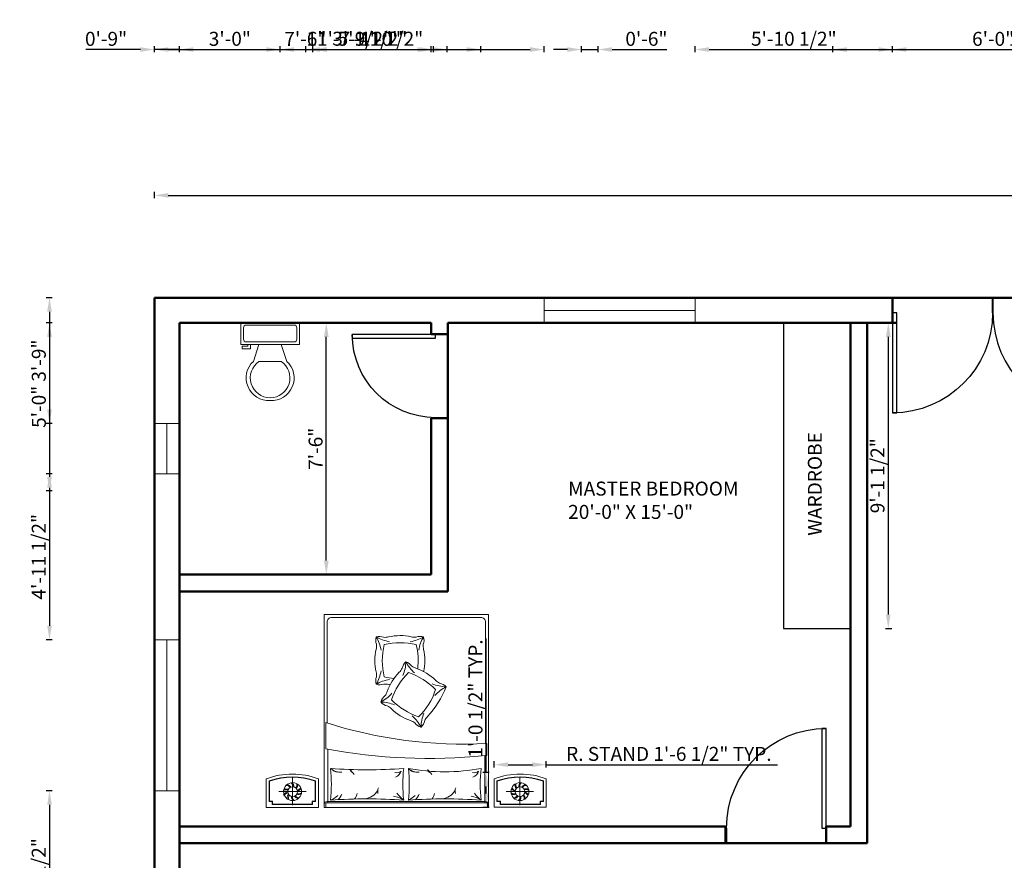
# Model space of a CAD drawing. Units: inches. Extents: x -46 to 764, y -530 to 112.
# Tile 2 of 5: x -46 to 307, y -188 to 112. Entities that reach past the tile are written whole.
import ezdxf

# ---------------------------------------------------------------- set-up
doc = ezdxf.new("R2010")
doc.units = ezdxf.units.IN
for name, color, linetype, lineweight in [('A-ANNO-DIMS', 2, 'Continuous', 18), ('A-AREA-IDEN', 7, 'Continuous', 18), ('A-DOOR', 3, 'Continuous', 25), ('A-FLOR-CASE', 32, 'Continuous', 25), ('A-FLOR-FIXT', 8, 'Continuous', 18), ('A-GLAZ', 4, 'Continuous', 18), ('A-WALL', 7, 'Continuous', 50), ('furn', 28, 'Continuous', 18), ('txt', 167, 'Continuous', 18)]:
    doc.layers.add(name, color=color, linetype=linetype, lineweight=lineweight)
doc.styles.get("Standard").update_dxf_attribs({"font": 'arial.ttf'})
doc.dimstyles.new('ISO-25', dxfattribs={"dimtxt": 5, "dimasz": 5, "dimexe": 1.25, "dimexo": 0.625, "dimtad": 1, "dimlunit": 3, "dimtxsty": 'Standard', "dimcen": 2.5, "dimadec": 0, "dimazin": 0, "dimtfac": 1, "dimtmove": 0, "dimatfit": 3, "dimfxl": 1, "dimfxlon": 1, "dimarcsym": 0})

# ---------------------------------------------------------------- blocks, each defined once
blk = doc.blocks.new('*U2')
for p, q in [((0, 0), (0, -6)), ((40, 0), (40, -6))]:
    blk.add_line(p, q)
blk.add_lwpolyline([(0, 0), (0, 40), (1.75, 40), (1.75, 0)], close=True)
blk.add_arc((0, 0), 40, 0, 90)
blk = doc.blocks.new('*U4')
for p, q in [((9.5, -6), (9.5, -2)), ((-10, -8.5), (-8, -8.5)), ((-10, -9.5), (-10, -8.5)), ((-7, -9.5), (-10, -9.5)), ((-8, -8.5), (-8, -8)), ((-7, -8), (-7, -9.5)), ((-4, -8), (-6, -14)), ((4, -8), (6, -14)), ((4, -14), (-4, -14))]:
    blk.add_line(p, q)
blk.add_lwpolyline([(10.5, -8), (10.5, 0), (-10.5, 0), (-10.5, -8)], close=True)
for points in [[(-9.5, -2), (-9.5, -6)], [(8.5, -1), (-8.5, -1)], [(-8.5, -7), (8.5, -7)]]:
    blk.add_lwpolyline(points)
for centre, radius, start, end in [((-8.625, -1.875), 0.8839, 81.8699, 188.1301), ((8.625, -1.875), 0.8839, 351.8699, 98.1301), ((-8.625, -6.125), 0.8839, 171.869898, 278.1301), ((8.625, -6.125), 0.8839, 261.8699, 8.1301), ((-0.4772, -19.9188), 8.0953, 133.01722, 273.38), ((0.0374, -19.8731), 7.127, 124.50543, 269.7), ((-0.0373, -19.8731), 7.127, 270.3, 55.4946), ((0.4773, -19.9188), 8.0953, 266.62, 46.9828)]:
    blk.add_arc(centre, radius, start, end)
blk = doc.blocks.new('*D10')
at = {"layer": 'A-ANNO-DIMS', "color": 0, "lineweight": -2, "transparency": 16777216}
for p, q in [((2.62, 48.57), (2.62, 50.82)), ((7.62, 49.57), (717.62, 49.57)), ((722.62, 48.57), (722.62, 50.82))]:
    blk.add_line(p, q, dxfattribs=at)
at = {"layer": 'A-ANNO-DIMS', "color": 0, "transparency": 16777216}
for points in [[(7.62, 50.4), (7.62, 48.73), (2.62, 49.57)], [(717.62, 50.4), (717.62, 48.73), (722.62, 49.57)]]:
    blk.add_solid(points, dxfattribs=at)
at = {"layer": 'Defpoints', "color": 0, "transparency": 16777216}
for p in [(722.62, 49.57), (2.62, 12.97), (722.62, 12.97)]:
    blk.add_point(p, dxfattribs=at)
at = {"layer": 'A-ANNO-DIMS', "color": 0, "transparency": 16777216, "insert": (362.62, 52.74), "char_height": 5, "attachment_point": 5}
blk.add_mtext("60'", dxfattribs=at)
blk = doc.blocks.new('BED-DOUBLE')
for p, q in [((1.34, 1.59), (1.34, 20.76)), ((57.43, 1.59), (57.43, 18.55)), ((57.72, 2.1), (1.02, 2.1))]:
    blk.add_line(p, q)
for points in [[(58.74, 0), (58.74, 68.93), (0, 68.93), (0, 0)], [(0.55, 0), (0.55, 1.59), (58.4, 1.59), (58.4, 0), (0, 0)]]:
    blk.add_lwpolyline(points)
for points in [[(57.72, 22.84), (57.72, 66.21, 0.414214), (56.03, 67.91), (2.72, 67.91, 0.414214), (1.02, 66.21), (1.02, 30.17)], [(18.6, 60.97, 0.159461), (18.72, 58.3, -0.076283), (18.6, 56.51, 0.115075), (18.6, 48.45, -0.076283), (18.72, 46.67, 0.159461), (18.6, 43.99)], [(20.35, 56.21, 0.091296), (18.6, 60.97, 0.091296), (23.37, 59.23)], [(30.8, 59.23, 0.091296), (35.58, 60.97, 0.091296), (33.82, 56.21, 0.091296)], [(32.9, 58.2, 0.111006), (21.48, 58.19, 0.119549), (21.48, 46.63, 0.033212), (24.99, 46.09)], [(29.21, 52.07, 0.159461), (27.9, 49.74, -0.076283), (26.85, 48.29, 0.115075), (22.59, 41.45, -0.076283), (21.75, 39.87, 0.159461), (20.23, 37.66)], [(28.18, 47.1, 0.091296), (29.21, 52.07, 0.091296), (32.34, 48.07)], [(23.37, 45.73, 0.091296), (18.6, 43.99, 0.091296), (20.35, 48.76, 0.091296)], [(39.88, 42.16, 0.111006), (30.18, 48.19, 0.119549), (24.07, 38.38, 0.107813), (33.74, 32.32)], [(38.65, 44.14, 0.091296), (43.62, 43.09, 0.091296), (39.61, 39.98, 0.091296)], [(25.2, 36.61, 0.091296), (20.23, 37.66, 0.091296), (24.24, 40.78, 0.091296)], [(33.79, 32.33, 0.121865), (39.88, 42.16, 0.121865)], [(35.68, 33.66, 0.091296), (34.64, 28.68, 0.091296), (31.51, 32.68, 0.091296)]]:
    blk.add_lwpolyline(points, format="xyb")
for points in [[(58.23, 18.55), (57.43, 18.55, -0.072944), (0.55, 20.92), (0.55, 30.34, 0.092568), (58.23, 22.87)], [(28.45, 13.91, 0.058596), (28.45, 2.57, 0.036648), (2.28, 2.57, 0.052163), (2.28, 13.91, 0.036967)], [(56.14, 13.91, 0.058596), (56.14, 2.57, 0.036889), (30.14, 2.57, 0.052163), (30.14, 13.91, 0.093111)]]:
    blk.add_lwpolyline(points, format="xyb", close=True)
for centre, radius, start, end in [((19.65, 56.16), 4.92, 70.7023, 102.284), ((21.76, 66.68), 5.9, 265.2252, 282.6741), ((27.14, 43.67), 17.74, 77.0576, 103.3153), ((32.37, 66.72), 5.9, 257.6988, 275.1477), ((34.43, 56.82), 4.3, 74.5791, 110.8198), ((31.43, 59.81), 4.3, 339.3666, 15.6073), ((9.55, 52.37), 24.07, 353.1956, 14.0284), ((41.33, 57.79), 5.9, 175.0387, 192.4877), ((18.3, 52.48), 17.74, 346.8711, 13.1289), ((27.56, 47.43), 4.92, 38.7754, 70.3571), ((34.92, 55.25), 5.9, 233.2983, 250.7472), ((27.31, 32.87), 17.74, 45.1307, 71.3884), ((19.87, 47.76), 3.97, 251.3996, 291.5774), ((21.86, 38.19), 5.9, 77.6988, 95.1477), ((27.09, 61.25), 17.74, 257.0576, 258.7033), ((9.2, 57.16), 37.18, 318.3818, 337.7644), ((43.94, 49.66), 5.9, 225.7718, 243.2208), ((40.46, 40.18), 4.3, 42.6522, 78.8929), ((23.3, 40.19), 3.97, 219.4726, 259.6505), ((19.93, 31.02), 5.9, 45.7718, 63.2208), ((36.56, 47.81), 17.74, 225.1307, 251.3884), ((41.21, 28.34), 5.9, 135.5854, 153.0343), ((28.95, 25.44), 5.9, 53.2983, 70.7472), ((35.78, 32.68), 4.15, 217.2937, 254.0973), ((31.74, 31.86), 4.3, 312.4658, 348.7065), ((4.9, 15.54), 2.94, 213.6349, 270.8456), ((5.76, 17.16), 4.64, 224.406, 276.8342), ((10.31, 13.43), 0.952, 173.7543, 257.2187), ((20.8, 21.81), 14.18, 216.2085, 225.0849), ((25.94, 14.96), 2.58, 256.4823, 308.5563), ((23.98, 14.17), 3.77, 294.2916, 340.9896), ((33.45, 17.16), 4.64, 224.406, 276.8342), ((32.59, 15.54), 2.94, 213.6349, 270.8456), ((38, 13.43), 0.952, 173.7543, 257.2187), ((48.49, 21.81), 14.18, 216.2085, 225.0849), ((53.63, 14.96), 2.58, 256.4823, 308.5563), ((51.67, 14.17), 3.77, 294.2916, 340.9896), ((-1.12, 10.34), 8.56, 294.6457, 314.1585), ((1.84, 6.34), 4.75, 310.5354, 340.3558), ((7.42, 5.72), 4.41, 321.8174, 349.8987), ((13.79, 9.29), 6.29, 276.6849, 328.3182), ((21.96, 5.79), 2.82, 155.8927, 196.1192), ((22.41, -6.92), 11.24, 57.5379, 77.5233), ((36.96, 13.18), 13.6, 216.4935, 231.2792), ((26.57, 10.34), 8.56, 294.6457, 314.1585), ((29.53, 6.34), 4.75, 310.5354, 340.3558), ((35.11, 5.72), 4.41, 321.8174, 349.8987), ((41.48, 9.29), 6.29, 276.6849, 328.3182), ((49.65, 5.79), 2.82, 155.8927, 196.1192), ((50.1, -6.92), 11.24, 57.5379, 77.5233), ((64.65, 13.18), 13.6, 216.4935, 231.2792), ((1.02, 1.08), 1.02, 90, 180), ((57.72, 1.08), 1.02, 0, 90)]:
    blk.add_arc(centre, radius, start, end)
blk = doc.blocks.new('NIGHTSTAND-L')
for p, q in [((9.43, 10.52), (9.43, 0.73)), ((4.54, 5.63), (14.33, 5.63))]:
    blk.add_line(p, q)
blk.add_lwpolyline([(0, 10.19), (0, 0), (18.68, 0), (18.68, 10.19, 0.181818)], format="xyb", close=True)
for points in [[(17.66, 2.14), (17.66, 9.48, 0.167087), (1.02, 9.48), (1.02, 2.14)], [(17.55, 2.14), (17.55, 9.4, 0.165559), (1.12, 9.4), (1.12, 2.14)]]:
    blk.add_lwpolyline(points, format="xyb")
for points in [[(2.24, 1.02), (2.24, 2.24), (1.02, 2.24)], [(2.14, 1.02), (2.14, 2.14), (1.02, 2.14)], [(2.14, 1.12), (16.54, 1.12)], [(2.14, 1.02), (16.54, 1.02)], [(16.43, 1.02), (16.43, 2.24), (17.66, 2.24)], [(16.54, 1.02), (16.54, 2.14), (17.66, 2.14)]]:
    blk.add_lwpolyline(points)
for radius in [3.2, 1.73]:
    blk.add_circle((9.43, 5.63), radius)
for centre, radius, start, end in [((7.17, 6.28), 1.57, 31.462, 91.6998), ((7.07, 6.1), 2.05, 33.5103, 79.83), ((7.98, 7.48), 1.57, 355.462, 55.6998), ((7.8, 7.4), 2.05, 357.5103, 43.83), ((9.35, 7.98), 1.57, 319.462, 19.6998), ((9.15, 8.02), 2.05, 321.5103, 7.83), ((10.75, 7.58), 1.57, 283.462, 343.6998), ((6.99, 4.73), 1.57, 67.462, 127.6998), ((7.01, 4.53), 2.05, 69.5103, 115.83), ((8.02, 3.43), 2.05, 105.5103, 151.83), ((7.89, 3.59), 1.57, 103.462, 163.6998), ((9.48, 3.14), 2.05, 141.5103, 187.83), ((9.52, 3.28), 1.57, 139.462, 199.6998), ((11.07, 3.86), 2.05, 177.5103, 223.83), ((10.88, 3.77), 1.57, 175.462, 235.6998), ((11.8, 5.16), 2.05, 213.5103, 259.83), ((11.7, 4.98), 1.57, 211.462, 271.6998), ((11.63, 6.64), 2.05, 249.5103, 295.83), ((11.64, 6.43), 1.57, 247.462, 307.6998), ((10.61, 7.73), 2.05, 285.5103, 331.83)]:
    blk.add_arc(centre, radius, start, end)
blk = doc.blocks.new('NIGHTSTAND-R')
for p, q in [((9.24, 10.52), (9.24, 0.73)), ((14.14, 5.62), (4.35, 5.62))]:
    blk.add_line(p, q)
blk.add_lwpolyline([(18.68, 10.19), (18.68, 0), (0, 0), (0, 10.19, -0.181818)], format="xyb", close=True)
for points in [[(1.02, 2.14), (1.02, 9.48, -0.167087), (17.66, 9.48), (17.66, 2.14)], [(1.12, 2.14), (1.12, 9.4, -0.165559), (17.56, 9.4), (17.56, 2.14)]]:
    blk.add_lwpolyline(points, format="xyb")
for points in [[(2.24, 1.02), (2.24, 2.24), (1.02, 2.24)], [(2.14, 1.02), (2.14, 2.14), (1.02, 2.14)], [(16.54, 1.12), (2.14, 1.12)], [(16.54, 1.02), (2.14, 1.02)], [(16.43, 1.02), (16.43, 2.24), (17.66, 2.24)], [(16.54, 1.02), (16.54, 2.14), (17.66, 2.14)]]:
    blk.add_lwpolyline(points)
for radius in [3.2, 1.73]:
    blk.add_circle((9.24, 5.62), radius)
for centre, radius, start, end in [((7.93, 7.57), 1.57, 196.3002, 256.538), ((9.52, 8.02), 2.05, 172.17, 218.4897), ((9.32, 7.97), 1.57, 160.3002, 220.538), ((10.88, 7.4), 2.05, 136.17, 182.4897), ((10.69, 7.48), 1.57, 124.3002, 184.538), ((11.61, 6.09), 2.05, 100.17, 146.4897), ((11.5, 6.27), 1.57, 88.3002, 148.538), ((7.03, 6.43), 1.57, 232.3002, 292.538), ((7.05, 6.63), 2.05, 244.17, 290.4897), ((8.06, 7.73), 2.05, 208.17, 254.4897), ((6.98, 4.98), 1.57, 268.3002, 328.538), ((6.88, 5.15), 2.05, 280.17, 326.4897), ((7.79, 3.77), 1.57, 304.3002, 4.538), ((7.6, 3.85), 2.05, 316.17, 2.4897), ((9.16, 3.27), 1.57, 340.3002, 40.538), ((8.96, 3.23), 2.05, 352.17, 38.4897), ((11.43, 4.61), 2.05, 64.17, 110.4897), ((11.45, 4.82), 1.57, 52.3002, 112.538), ((10.56, 3.67), 1.57, 16.3002, 76.538), ((10.42, 3.52), 2.05, 28.17, 74.4897)]:
    blk.add_arc(centre, radius, start, end)
blk = doc.blocks.new('WIN-54IN')
blk.add_line((4.5, 54), (4.5, 0))
blk.add_lwpolyline([(0, 54), (9, 54), (9, 0), (0, 0)], close=True)
blk = doc.blocks.new('WIN-18IN')
blk.add_line((4.5, 18), (4.5, 0))
blk.add_lwpolyline([(0, 18), (9, 18), (9, 0), (0, 0)], close=True)
blk = doc.blocks.new('*D31')
at = {"layer": 'A-ANNO-DIMS', "color": 0, "lineweight": -2, "transparency": 16777216}
for p, q in [((124.13, -154.98), (124.13, -152.73)), ((129.13, -153.98), (137.81, -153.98)), ((142.81, -154.98), (142.81, -152.73)), ((142.81, -153.98), (225.47, -153.98))]:
    blk.add_line(p, q, dxfattribs=at)
at = {"layer": 'A-ANNO-DIMS', "color": 0, "transparency": 16777216}
for points in [[(129.13, -153.14), (129.13, -154.81), (124.13, -153.98)], [(137.81, -153.14), (137.81, -154.81), (142.81, -153.98)]]:
    blk.add_solid(points, dxfattribs=at)
at = {"layer": 'Defpoints', "color": 0, "transparency": 16777216}
for p in [(142.81, -153.98), (124.13, -156.78), (142.81, -156.78)]:
    blk.add_point(p, dxfattribs=at)
at = {"layer": 'A-ANNO-DIMS', "color": 0, "transparency": 16777216, "insert": (186.64, -150.77), "char_height": 5, "attachment_point": 5}
blk.add_mtext('R. STAND 1\'-6 1/2" TYP.', dxfattribs=at)
blk = doc.blocks.new('*D32')
at = {"layer": 'A-ANNO-DIMS', "color": 0, "lineweight": -2, "transparency": 16777216}
for p, q in [((121.33, -156.78), (121.33, -108.87)), ((122.33, -156.78), (120.08, -156.78)), ((121.33, -164.23), (121.33, -161.78)), ((122.33, -169.23), (120.08, -169.23))]:
    blk.add_line(p, q, dxfattribs=at)
at = {"layer": 'A-ANNO-DIMS', "color": 0, "transparency": 16777216}
for points in [[(120.5, -161.78), (122.16, -161.78), (121.33, -156.78)], [(120.5, -164.23), (122.16, -164.23), (121.33, -169.23)]]:
    blk.add_solid(points, dxfattribs=at)
at = {"layer": 'Defpoints', "color": 0, "transparency": 16777216}
for p in [(121.33, -156.78), (124.13, -156.78), (124.13, -169.23)]:
    blk.add_point(p, dxfattribs=at)
at = {"layer": 'A-ANNO-DIMS', "color": 0, "transparency": 16777216, "insert": (118.12, -130.32), "char_height": 5, "attachment_point": 5, "rotation": 90}
blk.add_mtext('1\'-0 1/2" TYP.', dxfattribs=at)
blk = doc.blocks.new('*D43')
at = {"layer": 'A-ANNO-DIMS', "color": 0, "lineweight": -2, "transparency": 16777216}
for p, q in [((227.62, -503.53), (227.62, -505.78)), ((251.62, -503.53), (251.62, -505.78)), ((232.62, -504.53), (246.62, -504.53))]:
    blk.add_line(p, q, dxfattribs=at)
at = {"layer": 'A-ANNO-DIMS', "color": 0, "transparency": 16777216}
for points in [[(232.62, -503.7), (232.62, -505.36), (227.62, -504.53)], [(246.62, -503.7), (246.62, -505.36), (251.62, -504.53)]]:
    blk.add_solid(points, dxfattribs=at)
at = {"layer": 'Defpoints', "color": 0, "transparency": 16777216}
for p in [(227.62, -105.31), (251.62, -105.31), (251.62, -504.53)]:
    blk.add_point(p, dxfattribs=at)
at = {"layer": 'A-ANNO-DIMS', "color": 0, "transparency": 16777216, "insert": (239.62, -501.35), "char_height": 5, "attachment_point": 5}
blk.add_mtext('2\'-0"', dxfattribs=at)
blk = doc.blocks.new('*D44')
at = {"layer": 'A-ANNO-DIMS', "color": 0, "lineweight": -2, "transparency": 16777216}
for p, q in [((264.12, 3.97), (266.37, 3.97)), ((265.12, -1.03), (265.12, -100.31)), ((264.12, -105.31), (266.37, -105.31))]:
    blk.add_line(p, q, dxfattribs=at)
at = {"layer": 'A-ANNO-DIMS', "color": 0, "transparency": 16777216}
for points in [[(264.29, -1.03), (265.96, -1.03), (265.12, 3.97)], [(264.29, -100.31), (265.96, -100.31), (265.12, -105.31)]]:
    blk.add_solid(points, dxfattribs=at)
at = {"layer": 'Defpoints', "color": 0, "transparency": 16777216}
for p in [(227.62, 3.97), (227.62, -105.31), (265.12, -105.31)]:
    blk.add_point(p, dxfattribs=at)
at = {"layer": 'A-ANNO-DIMS', "color": 0, "transparency": 16777216, "insert": (261.91, -50.67), "char_height": 5, "attachment_point": 5, "rotation": 90}
blk.add_mtext('9\'-1 1/2"', dxfattribs=at)
blk = doc.blocks.new('*D45')
at = {"layer": 'A-ANNO-DIMS', "color": 0, "lineweight": -2, "transparency": 16777216}
for p, q in [((11.62, 100.72), (11.62, 102.97)), ((101.62, 100.72), (101.62, 102.97)), ((16.62, 101.72), (96.62, 101.72))]:
    blk.add_line(p, q, dxfattribs=at)
at = {"layer": 'A-ANNO-DIMS', "color": 0, "transparency": 16777216}
for points in [[(16.62, 102.55), (16.62, 100.88), (11.62, 101.72)], [(96.62, 102.55), (96.62, 100.88), (101.62, 101.72)]]:
    blk.add_solid(points, dxfattribs=at)
at = {"layer": 'Defpoints', "color": 0, "transparency": 16777216}
for p in [(101.62, 101.72), (11.62, -86.03), (101.62, -86.03)]:
    blk.add_point(p, dxfattribs=at)
at = {"layer": 'A-ANNO-DIMS', "color": 0, "transparency": 16777216, "insert": (56.62, 104.89), "char_height": 5, "attachment_point": 5}
blk.add_mtext('7\'-6"', dxfattribs=at)
blk = doc.blocks.new('*D46')
at = {"layer": 'A-ANNO-DIMS', "color": 0, "lineweight": -2, "transparency": 16777216}
for p, q in [((65.12, 3.97), (62.87, 3.97)), ((64.12, -81.03), (64.12, -1.03)), ((65.12, -86.03), (62.87, -86.03))]:
    blk.add_line(p, q, dxfattribs=at)
at = {"layer": 'A-ANNO-DIMS', "color": 0, "transparency": 16777216}
for points in [[(63.29, -1.03), (64.96, -1.03), (64.12, 3.97)], [(63.29, -81.03), (64.96, -81.03), (64.12, -86.03)]]:
    blk.add_solid(points, dxfattribs=at)
at = {"layer": 'Defpoints', "color": 0, "transparency": 16777216}
for p in [(64.12, 3.97), (101.62, 3.97), (101.62, -86.03)]:
    blk.add_point(p, dxfattribs=at)
at = {"layer": 'A-ANNO-DIMS', "color": 0, "transparency": 16777216, "insert": (60.95, -41.03), "char_height": 5, "attachment_point": 5, "rotation": 90}
blk.add_mtext('7\'-6"', dxfattribs=at)
blk = doc.blocks.new('*D48')
at = {"layer": 'A-ANNO-DIMS', "color": 0, "lineweight": -2, "transparency": 16777216}
for p, q in [((-33.88, 3.97), (-36.13, 3.97)), ((-34.88, -1.03), (-34.88, -51.03)), ((-33.88, -56.03), (-36.13, -56.03))]:
    blk.add_line(p, q, dxfattribs=at)
at = {"layer": 'A-ANNO-DIMS', "color": 0, "transparency": 16777216}
for points in [[(-35.71, -1.03), (-34.04, -1.03), (-34.88, 3.97)], [(-35.71, -51.03), (-34.04, -51.03), (-34.88, -56.03)]]:
    blk.add_solid(points, dxfattribs=at)
at = {"layer": 'Defpoints', "color": 0, "transparency": 16777216}
for p in [(713.62, 3.97), (-34.88, -56.03), (713.62, -56.03)]:
    blk.add_point(p, dxfattribs=at)
at = {"layer": 'A-ANNO-DIMS', "color": 0, "transparency": 16777216, "insert": (-38.05, -26.03), "char_height": 5, "attachment_point": 5, "rotation": 90}
blk.add_mtext('5\'-0"', dxfattribs=at)
blk = doc.blocks.new('*D49')
at = {"layer": 'A-ANNO-DIMS', "color": 0, "lineweight": -2, "transparency": 16777216}
for p, q in [((2.62, 100.72), (2.62, 102.97)), ((142.03, 100.72), (142.03, 102.97)), ((7.62, 101.72), (137.03, 101.72))]:
    blk.add_line(p, q, dxfattribs=at)
at = {"layer": 'A-ANNO-DIMS', "color": 0, "transparency": 16777216}
for points in [[(7.62, 102.55), (7.62, 100.88), (2.62, 101.72)], [(137.03, 102.55), (137.03, 100.88), (142.03, 101.72)]]:
    blk.add_solid(points, dxfattribs=at)
at = {"layer": 'Defpoints', "color": 0, "transparency": 16777216}
for p in [(142.03, 101.72), (2.62, 12.97), (142.03, 12.97)]:
    blk.add_point(p, dxfattribs=at)
at = {"layer": 'A-ANNO-DIMS', "color": 0, "transparency": 16777216, "insert": (72.33, 104.93), "char_height": 5, "attachment_point": 5}
blk.add_mtext('11\'-7 1/2"', dxfattribs=at)
blk = doc.blocks.new('*D50')
at = {"layer": 'A-ANNO-DIMS', "color": 0, "lineweight": -2, "transparency": 16777216}
for p, q in [((196.03, 100.72), (196.03, 102.97)), ((266.62, 100.72), (266.62, 102.97)), ((201.03, 101.72), (261.62, 101.72))]:
    blk.add_line(p, q, dxfattribs=at)
at = {"layer": 'A-ANNO-DIMS', "color": 0, "transparency": 16777216}
for points in [[(201.03, 102.55), (201.03, 100.88), (196.03, 101.72)], [(261.62, 102.55), (261.62, 100.88), (266.62, 101.72)]]:
    blk.add_solid(points, dxfattribs=at)
at = {"layer": 'Defpoints', "color": 0, "transparency": 16777216}
for p in [(266.62, 101.72), (196.03, 12.97), (266.62, 12.97)]:
    blk.add_point(p, dxfattribs=at)
at = {"layer": 'A-ANNO-DIMS', "color": 0, "transparency": 16777216, "insert": (231.33, 104.93), "char_height": 5, "attachment_point": 5}
blk.add_mtext('5\'-10 1/2"', dxfattribs=at)
blk = doc.blocks.new('*D51')
at = {"layer": 'A-ANNO-DIMS', "color": 0, "lineweight": -2, "transparency": 16777216}
for p, q in [((266.62, 100.72), (266.62, 102.97)), ((338.62, 100.72), (338.62, 102.97)), ((271.62, 101.72), (333.62, 101.72))]:
    blk.add_line(p, q, dxfattribs=at)
at = {"layer": 'A-ANNO-DIMS', "color": 0, "transparency": 16777216}
for points in [[(271.62, 102.55), (271.62, 100.88), (266.62, 101.72)], [(333.62, 102.55), (333.62, 100.88), (338.62, 101.72)]]:
    blk.add_solid(points, dxfattribs=at)
at = {"layer": 'Defpoints', "color": 0, "transparency": 16777216}
for p in [(338.62, 101.72), (266.62, 12.97), (338.62, 12.97)]:
    blk.add_point(p, dxfattribs=at)
at = {"layer": 'A-ANNO-DIMS', "color": 0, "transparency": 16777216, "insert": (302.62, 104.89), "char_height": 5, "attachment_point": 5}
blk.add_mtext('6\'-0"', dxfattribs=at)
blk = doc.blocks.new('*D53')
at = {"layer": 'A-ANNO-DIMS', "color": 0, "lineweight": -2, "transparency": 16777216}
for p, q in [((-33.88, 12.97), (-36.13, 12.97)), ((-34.88, 7.97), (-34.88, -26.97)), ((-33.88, -31.97), (-36.13, -31.97))]:
    blk.add_line(p, q, dxfattribs=at)
at = {"layer": 'A-ANNO-DIMS', "color": 0, "transparency": 16777216}
for points in [[(-35.71, 7.97), (-34.04, 7.97), (-34.88, 12.97)], [(-35.71, -26.97), (-34.04, -26.97), (-34.88, -31.97)]]:
    blk.add_solid(points, dxfattribs=at)
at = {"layer": 'Defpoints', "color": 0, "transparency": 16777216}
for p in [(2.62, 12.97), (-34.88, -31.97), (2.62, -31.97)]:
    blk.add_point(p, dxfattribs=at)
at = {"layer": 'A-ANNO-DIMS', "color": 0, "transparency": 16777216, "insert": (-38.06, -9.5), "char_height": 5, "attachment_point": 5, "rotation": 90}
blk.add_mtext('3\'-9"', dxfattribs=at)
blk = doc.blocks.new('*D54')
at = {"layer": 'A-ANNO-DIMS', "color": 0, "lineweight": -2, "transparency": 16777216}
for p, q in [((-33.88, -49.97), (-36.13, -49.97)), ((-34.88, -54.97), (-34.88, -104.31)), ((-33.88, -109.31), (-36.13, -109.31))]:
    blk.add_line(p, q, dxfattribs=at)
at = {"layer": 'A-ANNO-DIMS', "color": 0, "transparency": 16777216}
for points in [[(-35.71, -54.97), (-34.04, -54.97), (-34.88, -49.97)], [(-35.71, -104.31), (-34.04, -104.31), (-34.88, -109.31)]]:
    blk.add_solid(points, dxfattribs=at)
at = {"layer": 'Defpoints', "color": 0, "transparency": 16777216}
for p in [(2.62, -49.97), (-34.88, -109.31), (2.62, -109.31)]:
    blk.add_point(p, dxfattribs=at)
at = {"layer": 'A-ANNO-DIMS', "color": 0, "transparency": 16777216, "insert": (-38.09, -79.64), "char_height": 5, "attachment_point": 5, "rotation": 90}
blk.add_mtext('4\'-11 1/2"', dxfattribs=at)
blk = doc.blocks.new('*D55')
at = {"layer": 'A-ANNO-DIMS', "color": 0, "lineweight": -2, "transparency": 16777216}
for p, q in [((-33.88, -163.31), (-36.13, -163.31)), ((-34.88, -168.31), (-34.88, -219.03)), ((-33.88, -224.03), (-36.13, -224.03))]:
    blk.add_line(p, q, dxfattribs=at)
at = {"layer": 'A-ANNO-DIMS', "color": 0, "transparency": 16777216}
for points in [[(-35.71, -168.31), (-34.04, -168.31), (-34.88, -163.31)], [(-35.71, -219.03), (-34.04, -219.03), (-34.88, -224.03)]]:
    blk.add_solid(points, dxfattribs=at)
at = {"layer": 'Defpoints', "color": 0, "transparency": 16777216}
for p in [(2.62, -163.31), (-34.88, -224.03), (2.62, -224.03)]:
    blk.add_point(p, dxfattribs=at)
at = {"layer": 'A-ANNO-DIMS', "color": 0, "transparency": 16777216, "insert": (-38.09, -193.67), "char_height": 5, "attachment_point": 5, "rotation": 90}
blk.add_mtext('5\'-0 1/2"', dxfattribs=at)
blk = doc.blocks.new('*D68')
at = {"layer": 'A-ANNO-DIMS', "color": 0, "lineweight": -2, "transparency": 16777216}
for p, q in [((2.62, 100.72), (2.62, 102.97)), ((11.62, 100.72), (11.62, 102.97)), ((-2.38, 101.72), (-21.92, 101.72)), ((11.62, 101.72), (2.62, 101.72)), ((16.62, 101.72), (21.62, 101.72))]:
    blk.add_line(p, q, dxfattribs=at)
at = {"layer": 'A-ANNO-DIMS', "color": 0, "transparency": 16777216}
for points in [[(-2.38, 102.55), (-2.38, 100.88), (2.62, 101.72)], [(16.62, 102.55), (16.62, 100.88), (11.62, 101.72)]]:
    blk.add_solid(points, dxfattribs=at)
at = {"layer": 'Defpoints', "color": 0, "transparency": 16777216}
for p in [(2.62, 101.72), (11.62, -458.03), (2.62, -467.03)]:
    blk.add_point(p, dxfattribs=at)
at = {"layer": 'A-ANNO-DIMS', "color": 0, "transparency": 16777216, "insert": (-14.65, 104.89), "char_height": 5, "attachment_point": 5}
blk.add_mtext('0\'-9"', dxfattribs=at)
blk = doc.blocks.new('*D69')
at = {"layer": 'A-ANNO-DIMS', "color": 0, "lineweight": -2, "transparency": 16777216}
for p, q in [((155.34, 100.72), (155.34, 102.97)), ((161.34, 100.72), (161.34, 102.97)), ((150.34, 101.72), (145.34, 101.72)), ((155.34, 101.72), (161.34, 101.72)), ((166.34, 101.72), (185.88, 101.72))]:
    blk.add_line(p, q, dxfattribs=at)
at = {"layer": 'A-ANNO-DIMS', "color": 0, "transparency": 16777216}
for points in [[(150.34, 102.55), (150.34, 100.88), (155.34, 101.72)], [(166.34, 102.55), (166.34, 100.88), (161.34, 101.72)]]:
    blk.add_solid(points, dxfattribs=at)
at = {"layer": 'Defpoints', "color": 0, "transparency": 16777216}
for p in [(161.34, 101.72), (155.34, -458.03), (161.34, -458.03)]:
    blk.add_point(p, dxfattribs=at)
at = {"layer": 'A-ANNO-DIMS', "color": 0, "transparency": 16777216, "insert": (178.61, 104.89), "char_height": 5, "attachment_point": 5}
blk.add_mtext('0\'-6"', dxfattribs=at)
blk = doc.blocks.new('*D70')
at = {"layer": 'A-ANNO-DIMS', "color": 0, "lineweight": -2, "transparency": 16777216}
for p, q in [((59.34, 100.72), (59.34, 102.97)), ((107.34, 100.72), (107.34, 102.97)), ((64.34, 101.72), (102.34, 101.72))]:
    blk.add_line(p, q, dxfattribs=at)
at = {"layer": 'A-ANNO-DIMS', "color": 0, "transparency": 16777216}
for points in [[(64.34, 102.55), (64.34, 100.88), (59.34, 101.72)], [(102.34, 102.55), (102.34, 100.88), (107.34, 101.72)]]:
    blk.add_solid(points, dxfattribs=at)
at = {"layer": 'Defpoints', "color": 0, "transparency": 16777216}
for p in [(107.34, 101.72), (59.34, -308.03), (107.34, -308.03)]:
    blk.add_point(p, dxfattribs=at)
at = {"layer": 'A-ANNO-DIMS', "color": 0, "transparency": 16777216, "insert": (83.34, 104.89), "char_height": 5, "attachment_point": 5}
blk.add_mtext('4\'-0"', dxfattribs=at)
blk = doc.blocks.new('*D71')
at = {"layer": 'A-ANNO-DIMS', "color": 0, "lineweight": -2, "transparency": 16777216}
for p, q in [((47.62, 100.72), (47.62, 102.97)), ((119.34, 100.72), (119.34, 102.97)), ((52.62, 101.72), (114.34, 101.72))]:
    blk.add_line(p, q, dxfattribs=at)
at = {"layer": 'A-ANNO-DIMS', "color": 0, "transparency": 16777216}
for points in [[(52.62, 102.55), (52.62, 100.88), (47.62, 101.72)], [(114.34, 102.55), (114.34, 100.88), (119.34, 101.72)]]:
    blk.add_solid(points, dxfattribs=at)
at = {"layer": 'Defpoints', "color": 0, "transparency": 16777216}
for p in [(119.34, 101.72), (47.62, -422.03), (119.34, -422.03)]:
    blk.add_point(p, dxfattribs=at)
at = {"layer": 'A-ANNO-DIMS', "color": 0, "transparency": 16777216, "insert": (83.48, 104.93), "char_height": 5, "attachment_point": 5}
blk.add_mtext('5\'-11 1/2"', dxfattribs=at)
blk = doc.blocks.new('*D72')
at = {"layer": 'A-ANNO-DIMS', "color": 0, "lineweight": -2, "transparency": 16777216}
for p, q in [((11.62, 100.72), (11.62, 102.97)), ((47.62, 100.72), (47.62, 102.97)), ((16.62, 101.72), (42.62, 101.72))]:
    blk.add_line(p, q, dxfattribs=at)
at = {"layer": 'A-ANNO-DIMS', "color": 0, "transparency": 16777216}
for points in [[(16.62, 102.55), (16.62, 100.88), (11.62, 101.72)], [(42.62, 102.55), (42.62, 100.88), (47.62, 101.72)]]:
    blk.add_solid(points, dxfattribs=at)
at = {"layer": 'Defpoints', "color": 0, "transparency": 16777216}
for p in [(47.62, 101.72), (11.62, -363.17), (47.62, -363.17)]:
    blk.add_point(p, dxfattribs=at)
at = {"layer": 'A-ANNO-DIMS', "color": 0, "transparency": 16777216, "insert": (29.62, 104.9), "char_height": 5, "attachment_point": 5}
blk.add_mtext('3\'-0"', dxfattribs=at)
blk = doc.blocks.new('*D74')
at = {"layer": 'A-ANNO-DIMS', "color": 0, "lineweight": -2, "transparency": 16777216}
for p, q in [((56.83, 100.72), (56.83, 102.97)), ((102.5, 100.72), (102.5, 102.97)), ((61.83, 101.72), (97.5, 101.72))]:
    blk.add_line(p, q, dxfattribs=at)
at = {"layer": 'A-ANNO-DIMS', "color": 0, "transparency": 16777216}
for points in [[(61.83, 102.55), (61.83, 100.88), (56.83, 101.72)], [(97.5, 102.55), (97.5, 100.88), (102.5, 101.72)]]:
    blk.add_solid(points, dxfattribs=at)
at = {"layer": 'Defpoints', "color": 0, "transparency": 16777216}
for p in [(102.5, 101.72), (56.83, -426), (102.5, -426)]:
    blk.add_point(p, dxfattribs=at)
at = {"layer": 'A-ANNO-DIMS', "color": 0, "transparency": 16777216, "insert": (79.66, 104.93), "char_height": 5, "attachment_point": 5}
blk.add_mtext('3\'-9 1/2"', dxfattribs=at)
blk = doc.blocks.new('*D78')
at = {"layer": 'A-ANNO-DIMS', "color": 0, "lineweight": -2, "transparency": 16777216}
for p, q in [((245.34, 100.72), (245.34, 102.97)), ((401.62, 100.72), (401.62, 102.97)), ((250.34, 101.72), (396.62, 101.72))]:
    blk.add_line(p, q, dxfattribs=at)
at = {"layer": 'A-ANNO-DIMS', "color": 0, "transparency": 16777216}
for points in [[(250.34, 102.55), (250.34, 100.88), (245.34, 101.72)], [(396.62, 102.55), (396.62, 100.88), (401.62, 101.72)]]:
    blk.add_solid(points, dxfattribs=at)
at = {"layer": 'Defpoints', "color": 0, "transparency": 16777216}
for p in [(401.62, 101.72), (245.34, -458.03), (401.62, -458.03)]:
    blk.add_point(p, dxfattribs=at)
at = {"layer": 'A-ANNO-DIMS', "color": 0, "transparency": 16777216, "insert": (323.48, 104.93), "char_height": 5, "attachment_point": 5}
blk.add_mtext('13\'-0 1/2"', dxfattribs=at)
blk = doc.blocks.new('*D82')
at = {"layer": 'A-ANNO-DIMS', "color": 0, "lineweight": -2, "transparency": 16777216}
for p, q in [((33.53, -503.53), (33.53, -505.78)), ((54.53, -503.53), (54.53, -505.78)), ((38.53, -504.53), (49.53, -504.53))]:
    blk.add_line(p, q, dxfattribs=at)
at = {"layer": 'A-ANNO-DIMS', "color": 0, "transparency": 16777216}
for points in [[(38.53, -503.7), (38.53, -505.36), (33.53, -504.53)], [(49.53, -503.7), (49.53, -505.36), (54.53, -504.53)]]:
    blk.add_solid(points, dxfattribs=at)
at = {"layer": 'Defpoints', "color": 0, "transparency": 16777216}
for p in [(33.53, -3.78), (54.53, -3.78), (54.53, -504.53)]:
    blk.add_point(p, dxfattribs=at)
at = {"layer": 'A-ANNO-DIMS', "color": 0, "transparency": 16777216, "insert": (44.03, -501.35), "char_height": 5, "attachment_point": 5}
blk.add_mtext('1\'-9"', dxfattribs=at)
blk = doc.blocks.new('*D83')
at = {"layer": 'A-ANNO-DIMS', "color": 0, "lineweight": -2, "transparency": 16777216}
for p, q in [((759.12, 4.22), (761.37, 4.22)), ((760.12, -0.78), (760.12, -18.78)), ((759.12, -23.78), (761.37, -23.78))]:
    blk.add_line(p, q, dxfattribs=at)
at = {"layer": 'A-ANNO-DIMS', "color": 0, "transparency": 16777216}
for points in [[(759.29, -0.78), (760.96, -0.78), (760.12, 4.22)], [(759.29, -18.78), (760.96, -18.78), (760.12, -23.78)]]:
    blk.add_solid(points, dxfattribs=at)
at = {"layer": 'Defpoints', "color": 0, "transparency": 16777216}
for p in [(54.53, 4.22), (44.03, -23.78), (760.12, -23.78)]:
    blk.add_point(p, dxfattribs=at)
at = {"layer": 'A-ANNO-DIMS', "color": 0, "transparency": 16777216, "insert": (756.99, -9.78), "char_height": 5, "attachment_point": 5, "rotation": 90}
blk.add_mtext('2\'-4"', dxfattribs=at)

msp = doc.modelspace()

# ---------------------------------------------------------------- linework, layer by layer
at = {"layer": 'A-DOOR'}
msp.add_line((302.624, 5.473), (302.624, 12.97), dxfattribs=at)
at = {"layer": 'A-FLOR-CASE'}
for p, q in [((227.624, 3.97), (227.624, -105.31)), ((227.624, -105.31), (251.624, -105.31))]:
    msp.add_line(p, q, dxfattribs=at)
at = {"layer": 'A-WALL'}
for p, q in [((2.624, 12.97), (722.624, 12.97)), ((2.624, -467.03), (2.624, 12.97)), ((266.624, 3.97), (266.624, 12.97)), ((11.624, 3.97), (101.624, 3.97)), ((11.624, -224.03), (11.624, 3.97)), ((101.624, 3.97), (101.624, -0.03)), ((107.624, 3.97), (107.624, -92.03)), ((107.624, 3.97), (251.624, 3.97)), ((251.624, -176.03), (251.624, 3.97)), ((251.624, 3.97), (268.19, 3.97)), ((257.624, -182.03), (257.624, 3.97)), ((107.624, -0.03), (101.624, -0.03)), ((107.624, -30.03), (101.624, -30.03)), ((101.624, -30.03), (101.624, -86.03)), ((101.624, -86.03), (11.624, -86.03)), ((101.624, -92.03), (11.624, -92.03)), ((101.624, -92.03), (107.624, -92.03)), ((11.624, -176.03), (206.918, -176.03)), ((206.918, -176.03), (206.918, -182.03)), ((242.918, -176.03), (242.918, -182.03)), ((242.918, -176.03), (251.624, -176.03)), ((11.624, -182.03), (251.624, -182.03)), ((251.624, -182.03), (257.624, -182.03))]:
    msp.add_line(p, q, dxfattribs=at)

# ---------------------------------------------------------------- block references
at = {"layer": 'A-DOOR'}
for p, xscale, yscale, zscale, rotation in [((266.624, 7.602), -0.8946653133599701, 0.8946653133599701, 0.8946653133599701, 180), ((338.624, 7.561), 0.9015134452089247, 0.9015134452089247, 0.9015134452089247, 180), ((103.162, -0.159), -0.7436939408855294, 0.7436939408855294, 0.7436939408855294, 90)]:
    msp.add_blockref('*U2', p, dxfattribs=dict(at, xscale=xscale, yscale=yscale, zscale=zscale, rotation=rotation))
at = {"layer": 'A-DOOR', "xscale": -0.8915740545070651, "yscale": 0.8915740545070651, "zscale": 0.8915740545070651}
msp.add_blockref('*U2', (242.918, -176.68), dxfattribs=at)
at = {"layer": 'A-FLOR-FIXT'}
msp.add_blockref('*U4', (44.033, 4.216), dxfattribs=at)
at = {"layer": 'A-GLAZ', "rotation": 269.9999999999998}
msp.add_blockref('WIN-54IN', (142.032, 12.97), dxfattribs=at)
at = {"layer": 'A-GLAZ'}
for name, p in [('WIN-18IN', (2.624, -49.967)), ('WIN-54IN', (2.624, -163.312))]:
    msp.add_blockref(name, p, dxfattribs=at)
at = {"layer": 'furn'}
for name, p in [('BED-DOUBLE', (63.351, -169.232)), ('NIGHTSTAND-L', (42.638, -169.231)), ('NIGHTSTAND-R', (124.131, -169.228))]:
    msp.add_blockref(name, p, dxfattribs=at)

# ---------------------------------------------------------------- texts
at = {"layer": 'A-AREA-IDEN', "insert": (150.623, -52.767), "char_height": 5, "attachment_point": 1}
msp.add_mtext_dynamic_manual_height_columns('MASTER BEDROOM\\P20\'-0" X 15\'-0"', width=74.99503, gutter_width=12.5, heights=[0], dxfattribs=at)
at = {"layer": 'txt', "insert": (236.346, -72.136), "char_height": 5, "attachment_point": 1, "rotation": 90}
msp.add_mtext_dynamic_manual_height_columns('WARDROBE', width=154.75533, gutter_width=12.5, heights=[0], dxfattribs=at)

# ---------------------------------------------------------------- dimensions: what is measured, and where the dimension line sits
at = {"layer": 'A-ANNO-DIMS'}
for base, p1, p2, override, picture, middle in [((142.032, 101.716), (2.624, 12.97), (142.032, 12.97), {"dimdec": 1, "dimlfac": 1, "dimrnd": 0, "dimzin": 1, "dimdsep": 46, "dimlunit": 4, "dimfrac": 2}, '*D49', (72.328, 104.927)), ((119.339, 101.716), (47.624, -422.03), (119.339, -422.03), {"dimdec": 1, "dimlfac": 1, "dimrnd": 0, "dimzin": 1, "dimdsep": 46, "dimlunit": 4, "dimfrac": 2}, '*D71', (83.481, 104.927)), ((102.496, 101.716), (56.834, -426.004), (102.496, -426.004), {"dimdec": 1, "dimlfac": 1, "dimrnd": 0, "dimzin": 1, "dimdsep": 46, "dimlunit": 4, "dimfrac": 2}, '*D74', (79.665, 104.928)), ((266.624, 101.716), (196.032, 12.97), (266.624, 12.97), {"dimdec": 1, "dimlfac": 1, "dimrnd": 0, "dimzin": 1, "dimdsep": 46, "dimlunit": 4, "dimfrac": 2}, '*D50', (231.328, 104.927)), ((401.624, 101.716), (245.339, -458.03), (401.624, -458.03), {"dimdec": 1, "dimlfac": 1, "dimrnd": 0, "dimzin": 1, "dimdsep": 46, "dimlunit": 4, "dimfrac": 2}, '*D78', (323.481, 104.928)), ((2.624, 101.716), (11.624, -458.03), (2.624, -467.03), {"dimdec": 1, "dimlfac": 1, "dimrnd": 0, "dimzin": 1, "dimdsep": 46, "dimlunit": 4, "dimfrac": 2}, '*D68', (-14.646, 104.894)), ((47.624, 101.716), (11.624, -363.167), (47.624, -363.167), {"dimdec": 1, "dimlfac": 1, "dimrnd": 0, "dimzin": 1, "dimdsep": 46, "dimlunit": 4, "dimfrac": 2}, '*D72', (29.624, 104.896)), ((101.624, 101.716), (11.624, -86.03), (101.624, -86.03), {"dimdec": 1, "dimlfac": 1, "dimrnd": 0, "dimzin": 1, "dimdsep": 46, "dimlunit": 4, "dimfrac": 2}, '*D45', (56.624, 104.894)), ((107.339, 101.716), (59.339, -308.03), (107.339, -308.03), {"dimdec": 1, "dimlfac": 1, "dimrnd": 0, "dimzin": 1, "dimdsep": 46, "dimlunit": 4, "dimfrac": 2}, '*D70', (83.339, 104.894)), ((161.339, 101.716), (155.339, -458.03), (161.339, -458.03), {"dimdec": 1, "dimlfac": 1, "dimrnd": 0, "dimzin": 1, "dimdsep": 46, "dimlunit": 4, "dimfrac": 2}, '*D69', (178.609, 104.894)), ((338.624, 101.716), (266.624, 12.97), (338.624, 12.97), {"dimdec": 1, "dimlfac": 1, "dimrnd": 0, "dimzin": 1, "dimdsep": 46, "dimlunit": 4, "dimfrac": 2}, '*D51', (302.624, 104.894)), ((722.624, 49.565), (2.624, 12.97), (722.624, 12.97), {"dimclrd": 0, "dimclre": 0, "dimclrt": 0}, '*D10', (362.624, 52.743)), ((54.533, -504.53), (33.533, -3.784), (54.533, -3.784), {"dimdec": 1, "dimlfac": 1, "dimrnd": 0, "dimzin": 1, "dimdsep": 46, "dimlunit": 4, "dimfrac": 2}, '*D82', (44.033, -501.352)), ((251.624, -504.53), (227.624, -105.31), (251.624, -105.31), {"dimdec": 1, "dimlfac": 1, "dimrnd": 0, "dimzin": 1, "dimdsep": 46, "dimlunit": 4, "dimfrac": 2}, '*D43', (239.624, -501.352))]:
    dim = msp.add_linear_dim(base=base, p1=p1, p2=p2, dimstyle='ISO-25', override=override, dxfattribs=at)
    dim.commit()
    dim.dimension.update_dxf_attribs({"geometry": picture, "text_midpoint": middle})
for base, p1, p2, angle, picture, middle in [((-34.876, -31.966), (2.624, 12.97), (2.624, -31.966), 90, '*D53', (-38.055, -9.498)), ((-34.876, -56.03), (713.624, 3.97), (713.624, -56.03), 90, '*D48', (-38.054, -26.03)), ((760.124, -23.784), (54.533, 4.216), (44.033, -23.784), 90, '*D83', (756.989, -9.784)), ((64.124, 3.97), (101.624, -86.03), (101.624, 3.97), 90, '*D46', (60.946, -41.03)), ((265.124, -105.31), (227.624, 3.97), (227.624, -105.31), 270, '*D44', (261.914, -50.67)), ((-34.876, -109.312), (2.624, -49.966), (2.624, -109.312), 90, '*D54', (-38.086, -79.639)), ((-34.876, -224.03), (2.624, -163.312), (2.624, -224.03), 90, '*D55', (-38.086, -193.671))]:
    dim = msp.add_linear_dim(base=base, p1=p1, p2=p2, angle=angle, dimstyle='ISO-25', override={"dimdec": 1, "dimlfac": 1, "dimrnd": 0, "dimzin": 1, "dimdsep": 46, "dimlunit": 4, "dimfrac": 2}, dxfattribs=at)
    dim.commit()
    dim.dimension.update_dxf_attribs({"geometry": picture, "text_midpoint": middle})
dim = msp.add_linear_dim(base=(121.33, -156.777), p1=(124.131, -169.228), p2=(124.131, -156.777), angle=90, text='<> TYP.', dimstyle='ISO-25', override={"dimdec": 1, "dimlfac": 1, "dimrnd": 0, "dimzin": 1, "dimdsep": 46, "dimlunit": 4, "dimfrac": 2}, dxfattribs=at)
dim.commit()
dim.dimension.update_dxf_attribs({"geometry": '*D32', "text_midpoint": (118.12, -130.323)})
dim = msp.add_linear_dim(base=(142.807, -153.976), p1=(124.131, -156.777), p2=(142.807, -156.777), text='R. STAND <> TYP.', dimstyle='ISO-25', override={"dimdec": 1, "dimlfac": 1, "dimrnd": 0, "dimzin": 1, "dimdsep": 46, "dimlunit": 4, "dimfrac": 2}, dxfattribs=at)
dim.commit()
dim.dimension.update_dxf_attribs({"geometry": '*D31', "text_midpoint": (186.636, -150.766)})

doc.saveas('drawing.dxf')
